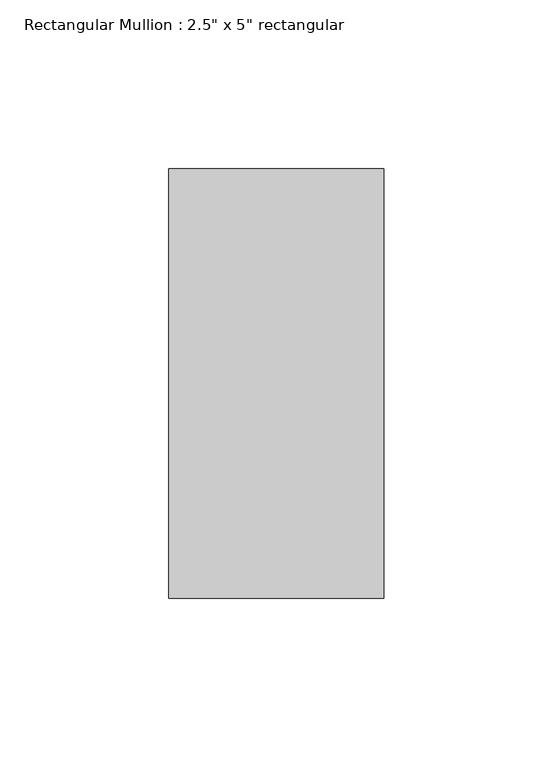
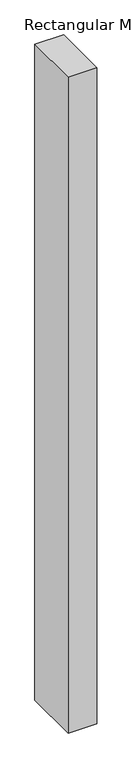
"""IFC4 building model written with IfcOpenShell, lengths in millimetres: member geometry."""

from ifc_helpers import new_model, si_unit, frame, origin, place, context, project, spatial, polyline, outline, extrude, source, transform, mapped, element, save


def member_0e7b3f94(model_context):
    return source(origin(), model_context, "Body", "SweptSolid", [
        extrude(outline(polyline([(31.75, 63.5), (31.75, -63.5), (-31.75, -63.5), (-31.75, 63.5), (31.75, 63.5)])), frame((0.0, 0.0, -1528.6649662), z_axis=(0.0, 0.0, 1.0), x_axis=(1.0, 0.0, 0.0)), (0.0, 0.0, 1.0), 1528.6649662),
    ])


if __name__ == "__main__":
    model = new_model("IFC4")
    model_context = context("Model", 3, world=origin())
    ifc_project = project(units=[si_unit("LENGTHUNIT", "METRE", prefix="MILLI")], contexts=[model_context])
    site = spatial("IfcSite", under=ifc_project)
    building = spatial("IfcBuilding", under=site)
    placement = place(None, origin())
    member_shape = member_0e7b3f94(model_context)
    element("IfcMember", 1, ObjectType="Rectangular Mullion : 2.5\" x 5\" rectangular", at=placement, inside=building, context=model_context, shape_type="MappedRepresentation", body=[
        mapped(member_shape, transform((0.0, 0.0, 0.0), x_axis=(1.0, 0.0, 0.0), y_axis=(0.0, 1.0, 0.0), z_axis=(0.0, 0.0, 1.0))),
    ])
    save(model, "model.ifc")

# Revit data of these elements
# Type "Rectangular Mullion : 2.5\" x 5\" rectangular"
#   built-in parameter 1007304 = 0.416667 (stored number, unit not read)
#   built-in parameter 1007301 = 0.104167 (stored number, unit not read)
#   built-in parameter 1007300 = 0.104167 (stored number, unit not read)
# Element 1 (IfcMember, "Rectangular Mullion : 2.5\" x 5\" rectangular")
#   Materials on its faces: "Aluminum"
# Materials
#   "Aluminum": class "Metal", colour RGB 247 247 247, transparency 0, Description = "Aluminum 6061", Cost = 0
